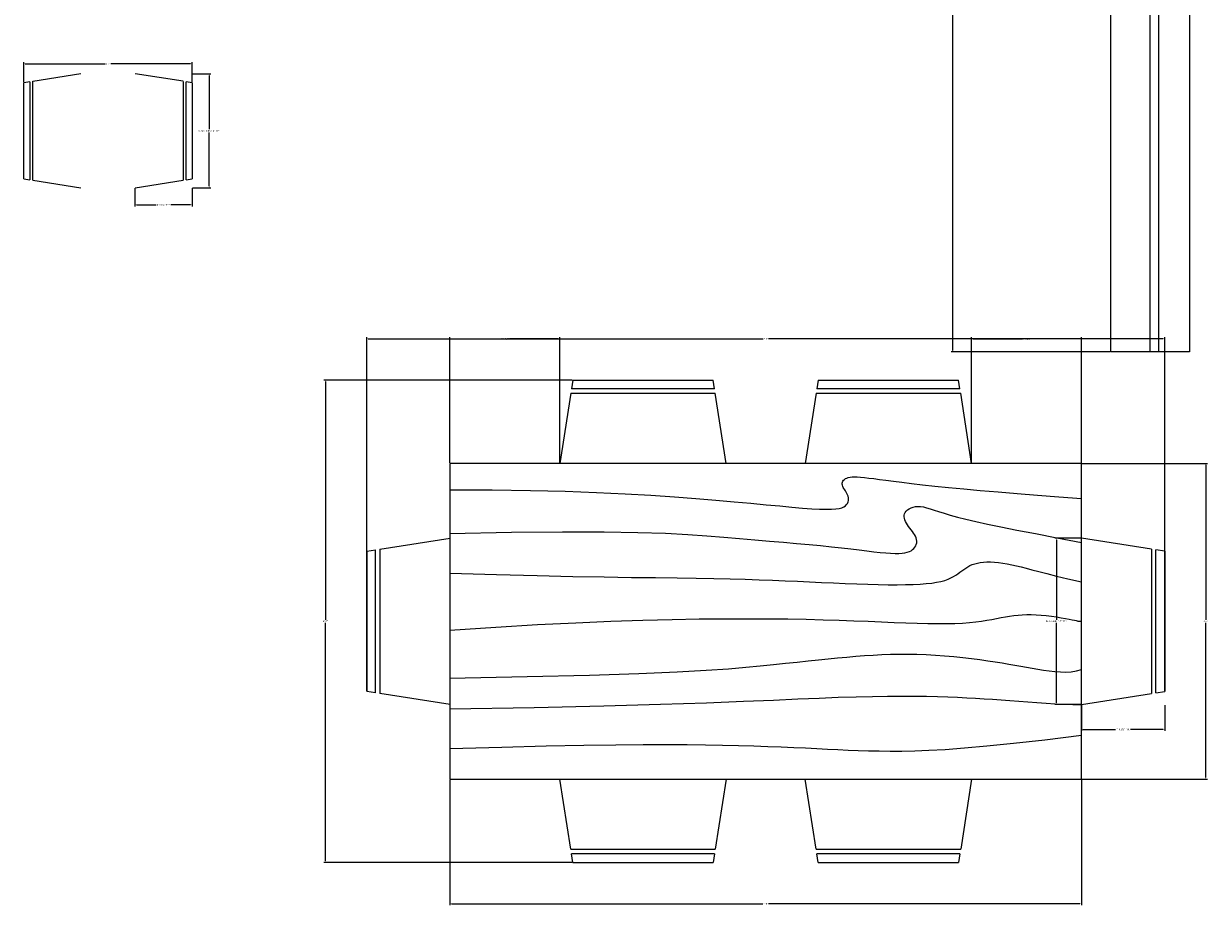
# Model space of a CAD drawing. Units: inches. Extents: x 226 to 1155, y 22 to 494.
# Tile 5 of 7: x 863 to 998, y 176 to 276. Entities that reach past the tile are written whole.
import ezdxf

# ---------------------------------------------------------------- set-up
doc = ezdxf.new("R2010")
doc.units = ezdxf.units.IN
doc.header["$MEASUREMENT"] = 0
for name, color, linetype, lineweight in [('A-ANNO-DIMS', 2, 'Continuous', 18), ('A-FURN', 8, 'Continuous', 18), ('A-GLAZ', 4, 'Continuous', 18)]:
    doc.layers.add(name, color=color, linetype=linetype, lineweight=lineweight)
doc.styles.get("Standard").update_dxf_attribs({"font": 'arial.ttf'})
doc.dimstyles.get("Standard").update_dxf_attribs({"dimtxt": 0.18, "dimasz": 0.18, "dimexe": 0.18, "dimexo": 0.0625, "dimgap": 0.09, "dimtad": 0, "dimtih": 1, "dimtoh": 1, "dimdec": 4, "dimzin": 0, "dimdsep": 46, "dimlunit": 4, "dimtxsty": 'Standard', "dimcen": 0.09, "dimadec": 0, "dimazin": 0, "dimtfac": 1, "dimtdec": 4, "dimtofl": 0, "dimtmove": 0, "dimatfit": 3, "dimfxl": 1, "dimtolj": 1, "dimtzin": 0, "dimarcsym": 0})

# ---------------------------------------------------------------- blocks, each defined once
blk = doc.blocks.new('CHAIR-DINING-FULL')
for p, q in [((1.48, 9.5), (1.33, 8.5)), ((1.48, 9.5), (17.48, 9.5)), ((17.64, 8.5), (17.48, 9.5)), ((17.64, 8.5), (1.33, 8.5)), ((1.25, 8), (0, 0)), ((1.25, 8), (17.72, 8)), ((18.97, 0), (17.72, 8))]:
    blk.add_line(p, q)
blk = doc.blocks.new('CHAIR-DINING-LINEAR')
for p, q in [((5.48, 12.14), (0, 12.99)), ((5.48, 12.13), (5.48, 0.85)), ((6.51, 11.98), (5.82, 12.08)), ((5.82, 0.91), (5.82, 12.08)), ((6.51, 11.98), (6.51, 1.02)), ((0, 0), (5.48, 0.86)), ((5.82, 0.91), (6.51, 1.02))]:
    blk.add_line(p, q)
blk = doc.blocks.new('WIN-120-SLIDING')
blk.add_lwpolyline([(9, 0), (0, 0), (0, 120), (9, 120)], close=True)
for points in [[(5.5, 0), (5.5, 60), (4.5, 60), (3.5, 60), (3.5, 120)], [(4.5, 0), (4.5, 60), (4.5, 120)]]:
    blk.add_lwpolyline(points)
blk = doc.blocks.new('*D26')
at = {"layer": 'A-ANNO-DIMS', "color": 0, "lineweight": -2, "transparency": 16777216}
for p, q in [((983.44, 217.49), (980.48, 217.49)), ((980.66, 217.31), (980.66, 208.19)), ((980.66, 198.7), (980.66, 207.82)), ((983.44, 198.52), (980.48, 198.52))]:
    blk.add_line(p, q, dxfattribs=at)
at = {"layer": 'A-ANNO-DIMS', "color": 0, "transparency": 16777216}
for points in [[(980.63, 217.31), (980.69, 217.31), (980.66, 217.49)], [(980.63, 198.7), (980.69, 198.7), (980.66, 198.52)]]:
    blk.add_solid(points, dxfattribs=at)
at = {"layer": 'Defpoints', "color": 0, "transparency": 16777216}
for p in [(983.51, 217.49), (980.66, 198.52), (983.51, 198.52)]:
    blk.add_point(p, dxfattribs=at)
at = {"layer": 'A-ANNO-DIMS', "color": 0, "transparency": 16777216, "insert": (980.66, 208.01), "char_height": 0.18, "attachment_point": 5}
blk.add_mtext('\\A1;END CHAIR 1\'-7" TYP.', dxfattribs=at)
blk = doc.blocks.new('*D27')
at = {"layer": 'A-ANNO-DIMS', "color": 0, "lineweight": -2, "transparency": 16777216}
for p, q in [((983.51, 198.46), (983.51, 195.5)), ((993.01, 198.46), (993.01, 195.5)), ((983.69, 195.68), (987.41, 195.68)), ((992.83, 195.68), (989.11, 195.68))]:
    blk.add_line(p, q, dxfattribs=at)
at = {"layer": 'A-ANNO-DIMS', "color": 0, "transparency": 16777216}
for points in [[(983.69, 195.71), (983.69, 195.65), (983.51, 195.68)], [(992.83, 195.71), (992.83, 195.65), (993.01, 195.68)]]:
    blk.add_solid(points, dxfattribs=at)
at = {"layer": 'Defpoints', "color": 0, "transparency": 16777216}
for p in [(983.51, 198.52), (993.01, 198.52), (993.01, 195.68)]:
    blk.add_point(p, dxfattribs=at)
at = {"layer": 'A-ANNO-DIMS', "color": 0, "transparency": 16777216, "insert": (988.26, 195.68), "char_height": 0.18, "attachment_point": 5}
blk.add_mtext('\\A1;0\'-9 1/2" TYP.', dxfattribs=at)
blk = doc.blocks.new('*D36')
at = {"layer": 'A-ANNO-DIMS', "color": 0, "lineweight": -2, "transparency": 16777216}
for p, q in [((882.16, 270.42), (884.23, 270.42)), ((884.05, 270.24), (884.05, 264.11)), ((884.05, 257.61), (884.05, 263.74)), ((882.16, 257.43), (884.23, 257.43))]:
    blk.add_line(p, q, dxfattribs=at)
at = {"layer": 'A-ANNO-DIMS', "color": 0, "transparency": 16777216}
for points in [[(884.02, 270.24), (884.08, 270.24), (884.05, 270.42)], [(884.02, 257.61), (884.08, 257.61), (884.05, 257.43)]]:
    blk.add_solid(points, dxfattribs=at)
at = {"layer": 'Defpoints', "color": 0, "transparency": 16777216}
for p in [(882.1, 270.42), (884.05, 270.42), (882.1, 257.43)]:
    blk.add_point(p, dxfattribs=at)
at = {"layer": 'A-ANNO-DIMS', "color": 0, "transparency": 16777216, "insert": (884.05, 263.93), "char_height": 0.18, "attachment_point": 5}
blk.add_mtext('\\A1;SIDE CHAIR 1\'-1" TYP.', dxfattribs=at)
blk = doc.blocks.new('*D37')
at = {"layer": 'A-ANNO-DIMS', "color": 0, "lineweight": -2, "transparency": 16777216}
for p, q in [((875.59, 257.37), (875.59, 255.3)), ((882.1, 257.37), (882.1, 255.3)), ((875.77, 255.48), (878, 255.48)), ((881.92, 255.48), (879.69, 255.48))]:
    blk.add_line(p, q, dxfattribs=at)
at = {"layer": 'A-ANNO-DIMS', "color": 0, "transparency": 16777216}
for points in [[(875.77, 255.51), (875.77, 255.45), (875.59, 255.48)], [(881.92, 255.51), (881.92, 255.45), (882.1, 255.48)]]:
    blk.add_solid(points, dxfattribs=at)
at = {"layer": 'Defpoints', "color": 0, "transparency": 16777216}
for p in [(875.59, 257.43), (882.1, 257.43), (882.1, 255.48)]:
    blk.add_point(p, dxfattribs=at)
at = {"layer": 'A-ANNO-DIMS', "color": 0, "transparency": 16777216, "insert": (878.85, 255.48), "char_height": 0.18, "attachment_point": 5}
blk.add_mtext('\\A1;0\'-6 1/2" TYP.', dxfattribs=at)
blk = doc.blocks.new('*D44')
at = {"layer": 'A-ANNO-DIMS', "color": 0, "lineweight": -2, "transparency": 16777216}
for p, q in [((986.79, 358.71), (968.67, 358.71)), ((968.85, 358.53), (968.85, 298.89)), ((968.85, 238.89), (968.85, 298.53)), ((986.79, 238.71), (968.67, 238.71))]:
    blk.add_line(p, q, dxfattribs=at)
at = {"layer": 'A-ANNO-DIMS', "color": 0, "transparency": 16777216}
for points in [[(968.82, 358.53), (968.88, 358.53), (968.85, 358.71)], [(968.82, 238.89), (968.88, 238.89), (968.85, 238.71)]]:
    blk.add_solid(points, dxfattribs=at)
at = {"layer": 'Defpoints', "color": 0, "transparency": 16777216}
for p in [(968.85, 358.71), (986.85, 358.71), (986.85, 238.71)]:
    blk.add_point(p, dxfattribs=at)
at = {"layer": 'A-ANNO-DIMS', "color": 0, "transparency": 16777216, "insert": (968.85, 298.71), "char_height": 0.18, "attachment_point": 5}
blk.add_mtext('\\A1;WINDOW 10\'-0" TYP.', dxfattribs=at)
blk = doc.blocks.new('*D95')
at = {"layer": 'A-ANNO-DIMS', "color": 0, "lineweight": -2, "transparency": 16777216}
for p, q in [((862.9, 269.47), (862.9, 271.75)), ((863.08, 271.57), (872.18, 271.57)), ((881.92, 271.57), (872.82, 271.57)), ((882.1, 269.47), (882.1, 271.75))]:
    blk.add_line(p, q, dxfattribs=at)
at = {"layer": 'A-ANNO-DIMS', "color": 0, "transparency": 16777216}
for points in [[(863.08, 271.6), (863.08, 271.54), (862.9, 271.57)], [(881.92, 271.6), (881.92, 271.54), (882.1, 271.57)]]:
    blk.add_solid(points, dxfattribs=at)
at = {"layer": 'Defpoints', "color": 0, "transparency": 16777216}
for p in [(882.1, 271.57), (862.9, 269.41), (882.1, 269.41)]:
    blk.add_point(p, dxfattribs=at)
at = {"layer": 'A-ANNO-DIMS', "color": 0, "transparency": 16777216, "insert": (872.5, 271.57), "char_height": 0.18, "attachment_point": 5}
blk.add_mtext('\\A1;1\'-7"', dxfattribs=at)
blk = doc.blocks.new('*D96')
at = {"layer": 'A-ANNO-DIMS', "color": 0, "lineweight": -2, "transparency": 16777216}
for p, q in [((902.01, 200.07), (902.01, 240.39)), ((902.19, 240.21), (947.18, 240.21)), ((992.83, 240.21), (947.84, 240.21)), ((993.01, 200.07), (993.01, 240.39))]:
    blk.add_line(p, q, dxfattribs=at)
at = {"layer": 'A-ANNO-DIMS', "color": 0, "transparency": 16777216}
for points in [[(902.19, 240.24), (902.19, 240.18), (902.01, 240.21)], [(992.83, 240.24), (992.83, 240.18), (993.01, 240.21)]]:
    blk.add_solid(points, dxfattribs=at)
at = {"layer": 'Defpoints', "color": 0, "transparency": 16777216}
for p in [(993.01, 240.21), (902.01, 200.01), (993.01, 200.01)]:
    blk.add_point(p, dxfattribs=at)
at = {"layer": 'A-ANNO-DIMS', "color": 0, "transparency": 16777216, "insert": (947.51, 240.21), "char_height": 0.18, "attachment_point": 5}
blk.add_mtext('\\A1;7\'-7"', dxfattribs=at)
blk = doc.blocks.new('*D97')
at = {"layer": 'A-ANNO-DIMS', "color": 0, "lineweight": -2, "transparency": 16777216}
for p, q in [((925.446854, 235.507939), (897.129352, 235.507939)), ((897.309352, 235.327939), (897.309352, 208.187937)), ((897.309352, 180.687935), (897.309352, 207.827937)), ((925.446854, 180.507935), (897.129352, 180.507935))]:
    blk.add_line(p, q, dxfattribs=at)
at = {"layer": 'A-ANNO-DIMS', "color": 0, "transparency": 16777216}
for points in [[(897.279352, 235.327939), (897.339352, 235.327939), (897.309352, 235.507939)], [(897.279352, 180.687935), (897.339352, 180.687935), (897.309352, 180.507935)]]:
    blk.add_solid(points, dxfattribs=at)
at = {"layer": 'Defpoints', "color": 0, "transparency": 16777216}
for p in [(897.309352, 235.507939), (925.509354, 235.507939), (925.509354, 180.507935)]:
    blk.add_point(p, dxfattribs=at)
at = {"layer": 'A-ANNO-DIMS', "color": 0, "transparency": 16777216, "insert": (897.309352, 208.007937), "char_height": 0.18, "attachment_point": 5}
blk.add_mtext('\\A1;4\'-7"', dxfattribs=at)
blk = doc.blocks.new('*D98')
at = {"layer": 'A-ANNO-DIMS', "color": 0, "lineweight": -2, "transparency": 16777216}
for p, q in [((911.51, 189.95), (911.51, 175.63)), ((983.51, 189.95), (983.51, 175.63)), ((911.69, 175.81), (947.18, 175.81)), ((983.33, 175.81), (947.84, 175.81))]:
    blk.add_line(p, q, dxfattribs=at)
at = {"layer": 'A-ANNO-DIMS', "color": 0, "transparency": 16777216}
for points in [[(911.69, 175.84), (911.69, 175.78), (911.51, 175.81)], [(983.33, 175.84), (983.33, 175.78), (983.51, 175.81)]]:
    blk.add_solid(points, dxfattribs=at)
at = {"layer": 'Defpoints', "color": 0, "transparency": 16777216}
for p in [(911.51, 190.01), (983.51, 190.01), (983.51, 175.81)]:
    blk.add_point(p, dxfattribs=at)
at = {"layer": 'A-ANNO-DIMS', "color": 0, "transparency": 16777216, "insert": (947.51, 175.81), "char_height": 0.18, "attachment_point": 5}
blk.add_mtext('\\A1;6\'-0"', dxfattribs=at)
blk = doc.blocks.new('*D99')
at = {"layer": 'A-ANNO-DIMS', "color": 0, "lineweight": -2, "transparency": 16777216}
for p, q in [((983.57, 226.01), (997.89, 226.01)), ((997.71, 225.83), (997.71, 208.19)), ((997.71, 190.19), (997.71, 207.83)), ((983.57, 190.01), (997.89, 190.01))]:
    blk.add_line(p, q, dxfattribs=at)
at = {"layer": 'A-ANNO-DIMS', "color": 0, "transparency": 16777216}
for points in [[(997.68, 225.83), (997.74, 225.83), (997.71, 226.01)], [(997.68, 190.19), (997.74, 190.19), (997.71, 190.01)]]:
    blk.add_solid(points, dxfattribs=at)
at = {"layer": 'Defpoints', "color": 0, "transparency": 16777216}
for p in [(983.51, 226.01), (997.71, 226.01), (983.51, 190.01)]:
    blk.add_point(p, dxfattribs=at)
at = {"layer": 'A-ANNO-DIMS', "color": 0, "transparency": 16777216, "insert": (997.71, 208.01), "char_height": 0.18, "attachment_point": 5}
blk.add_mtext('\\A1;3\'-0"', dxfattribs=at)
blk = doc.blocks.new('*D100')
at = {"layer": 'A-ANNO-DIMS', "color": 0, "lineweight": -2, "transparency": 16777216}
for p, q in [((911.51, 226.07), (911.51, 240.39)), ((911.69, 240.21), (917.24, 240.21)), ((923.84, 240.21), (918.3, 240.21)), ((924.02, 226.07), (924.02, 240.39))]:
    blk.add_line(p, q, dxfattribs=at)
at = {"layer": 'A-ANNO-DIMS', "color": 0, "transparency": 16777216}
for points in [[(911.69, 240.24), (911.69, 240.18), (911.51, 240.21)], [(923.84, 240.24), (923.84, 240.18), (924.02, 240.21)]]:
    blk.add_solid(points, dxfattribs=at)
at = {"layer": 'Defpoints', "color": 0, "transparency": 16777216}
for p in [(924.02, 240.21), (911.51, 226.01), (924.02, 226.01)]:
    blk.add_point(p, dxfattribs=at)
at = {"layer": 'A-ANNO-DIMS', "color": 0, "transparency": 16777216, "insert": (917.77, 240.21), "char_height": 0.18, "attachment_point": 5}
blk.add_mtext('\\A1;1\'-0 1/2"', dxfattribs=at)
blk = doc.blocks.new('*D101')
at = {"layer": 'A-ANNO-DIMS', "color": 0, "lineweight": -2, "transparency": 16777216}
for p, q in [((970.99, 226.07), (970.99, 240.39)), ((971.17, 240.21), (976.72, 240.21)), ((983.33, 240.21), (977.78, 240.21)), ((983.51, 226.07), (983.51, 240.39))]:
    blk.add_line(p, q, dxfattribs=at)
at = {"layer": 'A-ANNO-DIMS', "color": 0, "transparency": 16777216}
for points in [[(971.17, 240.24), (971.17, 240.18), (970.99, 240.21)], [(983.33, 240.24), (983.33, 240.18), (983.51, 240.21)]]:
    blk.add_solid(points, dxfattribs=at)
at = {"layer": 'Defpoints', "color": 0, "transparency": 16777216}
for p in [(983.51, 240.21), (970.99, 226.01), (983.51, 226.01)]:
    blk.add_point(p, dxfattribs=at)
at = {"layer": 'A-ANNO-DIMS', "color": 0, "transparency": 16777216, "insert": (977.25, 240.21), "char_height": 0.18, "attachment_point": 5}
blk.add_mtext('\\A1;1\'-0 1/2"', dxfattribs=at)

msp = doc.modelspace()

# ---------------------------------------------------------------- linework, layer by layer
at = {"layer": 'A-FURN'}
for p, q in [((983.50935, 226.00794), (911.50935, 226.00794)), ((911.50935, 226.00794), (911.50935, 190.00794)), ((983.50935, 190.00794), (983.50935, 226.00794)), ((911.50935, 190.00794), (983.50935, 190.00794))]:
    msp.add_line(p, q, dxfattribs=at)
for points in [[(911.50935, 223.00794), (916.33215, 222.98548), (920.70145, 222.922), (924.65555, 222.82337), (928.23335, 222.69544), (931.47315, 222.54407), (934.41365, 222.37512), (937.09345, 222.19446), (939.55105, 222.00794), (941.81895, 221.82109), (943.90585, 221.63815), (945.81395, 221.46302), (947.54585, 221.2996), (949.10385, 221.15182), (950.49045, 221.02356), (951.70815, 220.91874), (952.75935, 220.84127), (953.64865, 220.79407), (954.38955, 220.77617), (954.99765, 220.78561), (955.48855, 220.82044), (955.87785, 220.87871), (956.18125, 220.95846), (956.41425, 221.05774), (956.59265, 221.1746), (956.72985, 221.30693), (956.83095, 221.45195), (956.89885, 221.60673), (956.93645, 221.76835), (956.94665, 221.93388), (956.93255, 222.10039), (956.89685, 222.26494), (956.84265, 222.4246), (956.77315, 222.57711), (956.69295, 222.72278), (956.60685, 222.86259), (956.51975, 222.99752), (956.43655, 223.12854), (956.36225, 223.25664), (956.30155, 223.38277), (956.25935, 223.50794), (956.23985, 223.63261), (956.24375, 223.75533), (956.27105, 223.87415), (956.32185, 223.9871), (956.39605, 224.09225), (956.49375, 224.18762), (956.61485, 224.27128), (956.75935, 224.34127), (956.92825, 224.39596), (957.12655, 224.43502), (957.35995, 224.45846), (957.63435, 224.46627), (957.95565, 224.45846), (958.32965, 224.43502), (958.76225, 224.39596), (959.25935, 224.34127), (959.82775, 224.27112), (960.47875, 224.18632), (961.22445, 224.08785), (962.07705, 223.97669), (963.04885, 223.8538), (964.15195, 223.72018), (965.39865, 223.57678), (966.80105, 223.4246), (968.36835, 223.26461), (970.09725, 223.09778), (971.98145, 222.92509), (974.01455, 222.74752), (976.19025, 222.56604), (978.50225, 222.38164), (980.94405, 222.19527), (983.50935, 222.00794)], [(911.50935, 218.00794), (918.53275, 218.15068), (924.33685, 218.21236), (929.08525, 218.20569), (932.94165, 218.14335), (936.06945, 218.03805), (938.63235, 217.90247), (940.79395, 217.74931), (942.71765, 217.59127), (944.53955, 217.43876), (946.28475, 217.29309), (947.95085, 217.15328), (949.53535, 217.01835), (951.03595, 216.88733), (952.45015, 216.75924), (953.77535, 216.6331), (955.00935, 216.50794), (956.15045, 216.38343), (957.20075, 216.26184), (958.16315, 216.14612), (959.04055, 216.03919), (959.83605, 215.94397), (960.55235, 215.86341), (961.19245, 215.80042), (961.75935, 215.75794), (962.25645, 215.73824), (962.68905, 215.74101), (963.06305, 215.76526), (963.38435, 215.81002), (963.65875, 215.87431), (963.89215, 215.95716), (964.09045, 216.05758), (964.25935, 216.1746), (964.40375, 216.30709), (964.52365, 216.45325), (964.61825, 216.61113), (964.68645, 216.77877), (964.72735, 216.95423), (964.73985, 217.13554), (964.72305, 217.32076), (964.67605, 217.50794), (964.59885, 217.69544), (964.49635, 217.88294), (964.37425, 218.07044), (964.23855, 218.25794), (964.09495, 218.44544), (963.94945, 218.63294), (963.80785, 218.82044), (963.67605, 219.00794), (963.55935, 219.19527), (963.46115, 219.38164), (963.38455, 219.56604), (963.33225, 219.74752), (963.30735, 219.92509), (963.31275, 220.09778), (963.35135, 220.26461), (963.42605, 220.4246), (963.53885, 220.5763), (963.68775, 220.71627), (963.86985, 220.84062), (964.08225, 220.94544), (964.32205, 221.02682), (964.58615, 221.08085), (964.87185, 221.10364), (965.17605, 221.09127), (965.49875, 221.04106), (965.85115, 220.9552), (966.24755, 220.83712), (966.70205, 220.69023), (967.22885, 220.51795), (967.84205, 220.32369), (968.55585, 220.11088), (969.38435, 219.88294), (970.34505, 219.64148), (971.46835, 219.38098), (972.78795, 219.09412), (974.33755, 218.77356), (976.15075, 218.41199), (978.26135, 218.00208), (980.70295, 217.5365), (983.50935, 217.00794)], [(911.50935, 213.50794), (916.79365, 213.34274), (921.44035, 213.21757), (925.51475, 213.12561), (929.08225, 213.06002), (932.20845, 213.01396), (934.95855, 212.98059), (937.39815, 212.95309), (939.59265, 212.9246), (941.60035, 212.88961), (943.45075, 212.84778), (945.16645, 212.80009), (946.76975, 212.74752), (948.28325, 212.69104), (949.72935, 212.63164), (951.13065, 212.57027), (952.50935, 212.50794), (953.88235, 212.44576), (955.24375, 212.38554), (956.58165, 212.32923), (957.88435, 212.27877), (959.14025, 212.23613), (960.33745, 212.20325), (961.46445, 212.18209), (962.50935, 212.1746), (963.46335, 212.18242), (964.32835, 212.20585), (965.10945, 212.24492), (965.81145, 212.2996), (966.43925, 212.36992), (966.99765, 212.45585), (967.49165, 212.55742), (967.92605, 212.6746), (968.30625, 212.80693), (968.63955, 212.95195), (968.93385, 213.10673), (969.19685, 213.26835), (969.43645, 213.43388), (969.66045, 213.60039), (969.87655, 213.76494), (970.09275, 213.9246), (970.31585, 214.07662), (970.54975, 214.21887), (970.79725, 214.34941), (971.06145, 214.46627), (971.34515, 214.56751), (971.65135, 214.65117), (971.98285, 214.71529), (972.34275, 214.75794), (972.73285, 214.77763), (973.15135, 214.77486), (973.59515, 214.75061), (974.06145, 214.70585), (974.54725, 214.64156), (975.04975, 214.55872), (975.56585, 214.4583), (976.09275, 214.34127), (976.63355, 214.20781), (977.21645, 214.05481), (977.87545, 213.87838), (978.64475, 213.6746), (979.55865, 213.43958), (980.65135, 213.1694), (981.95685, 212.86015), (983.50935, 212.50794)], [(911.50935, 207.00794), (916.71785, 207.34884), (921.48985, 207.62578), (925.85745, 207.8451), (929.85305, 208.01315), (933.50885, 208.13627), (936.85705, 208.22083), (939.92975, 208.27316), (942.75935, 208.2996), (945.37535, 208.30587), (947.79715, 208.29505), (950.04105, 208.26957), (952.12395, 208.2319), (954.06225, 208.18445), (955.87265, 208.12968), (957.57165, 208.07003), (959.17605, 208.00794), (960.69925, 207.94593), (962.14345, 207.88684), (963.50755, 207.83362), (964.79065, 207.78919), (965.99165, 207.75647), (967.10965, 207.73841), (968.14365, 207.73792), (969.09275, 207.75794), (969.95745, 207.80026), (970.74505, 207.8621), (971.46425, 207.93958), (972.12395, 208.02877), (972.73285, 208.12578), (973.29975, 208.22669), (973.83345, 208.3276), (974.34275, 208.4246), (974.83585, 208.51412), (975.31925, 208.59387), (975.79875, 208.66191), (976.28025, 208.71627), (976.76945, 208.75501), (977.27235, 208.77617), (977.79485, 208.77779), (978.34275, 208.75794), (978.91815, 208.71578), (979.50875, 208.65507), (980.09835, 208.58069), (980.67085, 208.49752), (981.21015, 208.41044), (981.70015, 208.32434), (982.12465, 208.2441), (982.46775, 208.1746), (982.71925, 208.11959), (982.89415, 208.07825), (983.01335, 208.04863), (983.09795, 208.02877), (983.16875, 208.01673), (983.24705, 208.01054), (983.35355, 208.00826), (983.50935, 208.00794)], [(911.50935, 201.50794), (920.32505, 201.69527), (927.42535, 201.88164), (933.04035, 202.06604), (937.39995, 202.24752), (940.73415, 202.42509), (943.27305, 202.59778), (945.24645, 202.76461), (946.88435, 202.9246), (948.38015, 203.07695), (949.78085, 203.22148), (951.09655, 203.3582), (952.33745, 203.4871), (953.51395, 203.6082), (954.63635, 203.72148), (955.71465, 203.82695), (956.75935, 203.9246), (957.77985, 204.01412), (958.78275, 204.09387), (959.77405, 204.16191), (960.75935, 204.21627), (961.74475, 204.25501), (962.73595, 204.27617), (963.73885, 204.27779), (964.75935, 204.25794), (965.80055, 204.21546), (966.85445, 204.15247), (967.91025, 204.0719), (968.95725, 203.97669), (969.98475, 203.86975), (970.98205, 203.75403), (971.93825, 203.63245), (972.84275, 203.50794), (973.68785, 203.38302), (974.47875, 203.25859), (975.22385, 203.13513), (975.93125, 203.01315), (976.60935, 202.89311), (977.26655, 202.77552), (977.91095, 202.66085), (978.55105, 202.5496), (979.19305, 202.44357), (979.83555, 202.34973), (980.47515, 202.27641), (981.10835, 202.2319), (981.73175, 202.22449), (982.34205, 202.26249), (982.93575, 202.35421), (983.50935, 202.50794)], [(911.50935, 198.00794), (921.10715, 198.19495), (929.04185, 198.37903), (935.52545, 198.55725), (940.76975, 198.72669), (944.98675, 198.8844), (948.38825, 199.02747), (951.18625, 199.15296), (953.59265, 199.25794), (955.78605, 199.34029), (957.81145, 199.40117), (959.68055, 199.44251), (961.40515, 199.46627), (962.99695, 199.47441), (964.46765, 199.46887), (965.82905, 199.45162), (967.09275, 199.4246), (968.27095, 199.38953), (969.37785, 199.34713), (970.42815, 199.2979), (971.43645, 199.24231), (972.41745, 199.18087), (973.38565, 199.11406), (974.35585, 199.04236), (975.34275, 198.96627), (976.35675, 198.88676), (977.39215, 198.80677), (978.43935, 198.7297), (979.48855, 198.65898), (980.52985, 198.59803), (981.55365, 198.55026), (982.55005, 198.51909), (983.50935, 198.50794)], [(911.50935, 193.50794), (917.42125, 193.67281), (922.47615, 193.7957), (926.77815, 193.88147), (930.43125, 193.93502), (933.53935, 193.96123), (936.20665, 193.96497), (938.53695, 193.95113), (940.63435, 193.9246), (942.58695, 193.88961), (944.41885, 193.84778), (946.13845, 193.80009), (947.75415, 193.74752), (949.27405, 193.69104), (950.70665, 193.63164), (952.06005, 193.57027), (953.34265, 193.50794), (954.56475, 193.44584), (955.74435, 193.38619), (956.90155, 193.33142), (958.05625, 193.28398), (959.22855, 193.2463), (960.43835, 193.22083), (961.70585, 193.21), (963.05105, 193.21627), (964.50265, 193.2437), (966.12455, 193.30286), (967.98975, 193.40597), (970.17085, 193.56523), (972.74055, 193.79285), (975.77175, 194.10104), (979.33705, 194.502), (983.50935, 195.00794)]]:
    msp.add_lwpolyline(points, dxfattribs=at)

# ---------------------------------------------------------------- block references
for name, p, rotation in [('CHAIR-DINING-LINEAR', (869.4067, 270.42403), 180), ('CHAIR-DINING-FULL', (983.50742, 217.4923), 270)]:
    msp.add_blockref(name, p, dxfattribs=dict(at, rotation=rotation))
for name, p in [('CHAIR-DINING-LINEAR', (875.592, 257.43)), ('CHAIR-DINING-FULL', (924.025, 226.006)), ('CHAIR-DINING-FULL', (952.025, 226.006))]:
    msp.add_blockref(name, p, dxfattribs=at)
at = {"layer": 'A-FURN', "extrusion": (0, 0, -1), "zscale": -1}
for p, rotation in [((-911.51129, 217.4923), 270), ((-924.025, 190.00987), 180), ((-952.025, 190.00987), 180)]:
    msp.add_blockref('CHAIR-DINING-FULL', p, dxfattribs=dict(at, rotation=rotation))
at = {"layer": 'A-GLAZ'}
msp.add_blockref('WIN-120-SLIDING', (986.85159, 238.70877), dxfattribs=at)

# ---------------------------------------------------------------- dimensions: what is measured, and where the dimension line sits
at = {"layer": 'A-ANNO-DIMS'}
for base, p1, p2, angle, text, picture, middle in [((968.85144, 358.70847), (986.85144, 238.70847), (986.85144, 358.70847), 90, 'WINDOW <> TYP.', '*D44', (968.85144, 298.70847)), ((884.04969, 270.42359), (882.10072, 257.43044), (882.10072, 270.42359), 90, 'SIDE CHAIR <> TYP.', '*D36', (884.04969, 263.92702)), ((980.66156, 198.52314), (983.50698, 217.49264), (983.50698, 198.52314), 270, 'END CHAIR <> TYP.', '*D26', (980.66156, 208.00789))]:
    dim = msp.add_linear_dim(base=base, p1=p1, p2=p2, angle=angle, text=text, dimstyle='Standard', override={"dimdec": 1, "dimlfac": 1, "dimrnd": 0, "dimzin": 1, "dimdsep": 46, "dimlunit": 4, "dimfrac": 2}, dxfattribs=at)
    dim.commit()
    dim.dimension.update_dxf_attribs({"geometry": picture, "text_midpoint": middle})
for base, p1, p2, picture, middle in [((882.10072, 271.57359), (862.89798, 269.40658), (882.10072, 269.40665), '*D95', (872.49935, 271.57359)), ((924.02465, 240.20794), (911.50935, 226.00794), (924.02465, 226.00556), '*D100', (917.767, 240.20794)), ((983.50935, 240.20794), (970.99415, 226.00556), (983.50935, 226.00794), '*D101', (977.25175, 240.20794)), ((993.00936, 240.20794), (902.00935, 200.00794), (993.00936, 200.00794), '*D96', (947.50936, 240.20794)), ((983.50935, 175.80793), (911.50935, 190.00794), (983.50935, 190.00794), '*D98', (947.50935, 175.80793))]:
    dim = msp.add_linear_dim(base=base, p1=p1, p2=p2, dimstyle='Standard', override={"dimdec": 1, "dimlfac": 1, "dimrnd": 0, "dimzin": 1, "dimdsep": 46, "dimlunit": 4, "dimfrac": 2}, dxfattribs=at)
    dim.commit()
    dim.dimension.update_dxf_attribs({"geometry": picture, "text_midpoint": middle})
for base, p1, p2, picture, middle in [((882.10072, 255.48147), (875.59207, 257.43044), (882.10072, 257.43044), '*D37', (878.84639, 255.48147)), ((993.00936, 195.67772), (983.50698, 198.52314), (993.00936, 198.52314), '*D27', (988.25817, 195.67772))]:
    dim = msp.add_linear_dim(base=base, p1=p1, p2=p2, text='<> TYP.', dimstyle='Standard', override={"dimdec": 1, "dimlfac": 1, "dimrnd": 0, "dimzin": 1, "dimdsep": 46, "dimlunit": 4, "dimfrac": 2}, dxfattribs=at)
    dim.commit()
    dim.dimension.update_dxf_attribs({"geometry": picture, "text_midpoint": middle})
for base, p1, p2, picture, middle in [((897.30935, 235.50794), (925.50935, 180.50794), (925.50935, 235.50794), '*D97', (897.30935, 208.00794)), ((997.70936, 226.00794), (983.50935, 190.00794), (983.50935, 226.00794), '*D99', (997.70936, 208.00794))]:
    dim = msp.add_linear_dim(base=base, p1=p1, p2=p2, angle=90, dimstyle='Standard', override={"dimdec": 1, "dimlfac": 1, "dimrnd": 0, "dimzin": 1, "dimdsep": 46, "dimlunit": 4, "dimfrac": 2}, dxfattribs=at)
    dim.commit()
    dim.dimension.update_dxf_attribs({"geometry": picture, "text_midpoint": middle})

doc.saveas('drawing.dxf')
